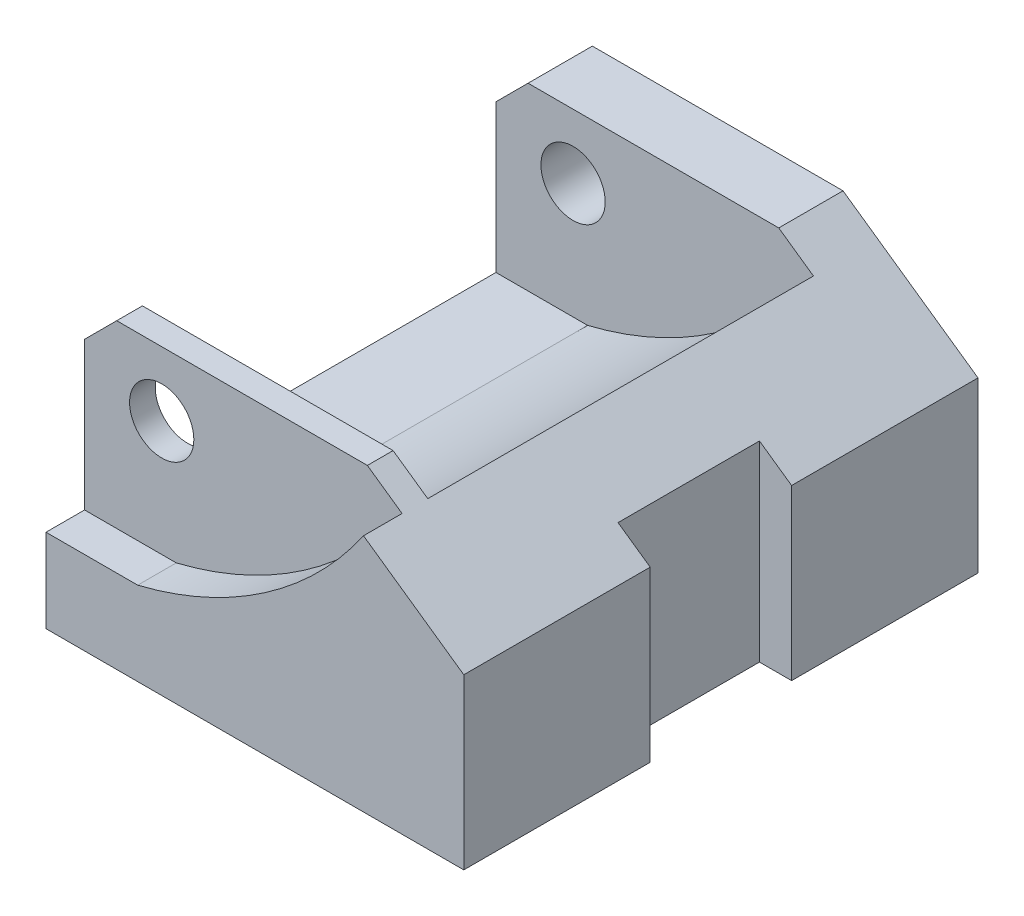
ISO-10303-21;
HEADER;
FILE_DESCRIPTION(('STEP AP214'),'2;1');
FILE_NAME('part.step','',(''),(''),'','','');
FILE_SCHEMA(('AUTOMOTIVE_DESIGN { 1 0 10303 214 1 1 1 1 }'));
ENDSEC;
DATA;
#1=APPLICATION_CONTEXT('core data for automotive mechanical design processes');
#2=APPLICATION_PROTOCOL_DEFINITION('international standard','automotive_design',2000,#1);
#3=PRODUCT_CONTEXT('',#1,'mechanical');
#4=PRODUCT('Part','Part','',(#3));
#5=PRODUCT_RELATED_PRODUCT_CATEGORY('part','',(#4));
#6=PRODUCT_DEFINITION_FORMATION('','',#4);
#7=PRODUCT_DEFINITION_CONTEXT('part definition',#1,'design');
#8=PRODUCT_DEFINITION('design','',#6,#7);
#9=PRODUCT_DEFINITION_SHAPE('','',#8);
#10=(LENGTH_UNIT() NAMED_UNIT(*) SI_UNIT(.MILLI.,.METRE.));
#11=(NAMED_UNIT(*) PLANE_ANGLE_UNIT() SI_UNIT($,.RADIAN.));
#12=(NAMED_UNIT(*) SI_UNIT($,.STERADIAN.) SOLID_ANGLE_UNIT());
#13=UNCERTAINTY_MEASURE_WITH_UNIT(LENGTH_MEASURE(1.E-05),#10,'distance_accuracy_value','');
#14=(GEOMETRIC_REPRESENTATION_CONTEXT(3) GLOBAL_UNCERTAINTY_ASSIGNED_CONTEXT((#13)) GLOBAL_UNIT_ASSIGNED_CONTEXT((#10,
#11,#12)) REPRESENTATION_CONTEXT('',''));
#15=CARTESIAN_POINT('',(0.,0.,0.));
#16=DIRECTION('',(0.,0.,1.));
#17=DIRECTION('',(1.,0.,0.));
#18=AXIS2_PLACEMENT_3D('',#15,#16,#17);
#19=CARTESIAN_POINT('',(65.,0.,40.));
#20=DIRECTION('',(-1.,0.,0.));
#21=DIRECTION('',(0.,0.,1.));
#22=AXIS2_PLACEMENT_3D('',#19,#20,#21);
#23=PLANE('',#22);
#24=DIRECTION('',(0.,-1.,0.));
#25=VECTOR('',#24,1.);
#26=CARTESIAN_POINT('',(65.,0.,11.));
#27=LINE('',#26,#25);
#28=CARTESIAN_POINT('',(65.,26.2956416975961,11.));
#29=VERTEX_POINT('',#28);
#30=CARTESIAN_POINT('',(65.,0.,11.));
#31=VERTEX_POINT('',#30);
#32=EDGE_CURVE('E176',#29,#31,#27,.T.);
#33=ORIENTED_EDGE('',*,*,#32,.F.);
#34=DIRECTION('',(0.,0.,1.));
#35=VECTOR('',#34,1.);
#36=CARTESIAN_POINT('',(65.,26.2956416975961,40.));
#37=LINE('',#36,#35);
#38=CARTESIAN_POINT('',(65.,26.2956416975961,40.));
#39=VERTEX_POINT('',#38);
#40=EDGE_CURVE('E319',#29,#39,#37,.T.);
#41=ORIENTED_EDGE('',*,*,#40,.T.);
#42=DIRECTION('',(0.,1.,0.));
#43=VECTOR('',#42,1.);
#44=CARTESIAN_POINT('',(65.,0.,40.));
#45=LINE('',#44,#43);
#46=CARTESIAN_POINT('',(65.,0.,40.));
#47=VERTEX_POINT('',#46);
#48=EDGE_CURVE('E288',#47,#39,#45,.T.);
#49=ORIENTED_EDGE('',*,*,#48,.F.);
#50=DIRECTION('',(0.,0.,-1.));
#51=VECTOR('',#50,1.);
#52=CARTESIAN_POINT('',(65.,0.,40.));
#53=LINE('',#52,#51);
#54=EDGE_CURVE('E298',#47,#31,#53,.T.);
#55=ORIENTED_EDGE('',*,*,#54,.T.);
#56=EDGE_LOOP('',(#33,#41,#49,#55));
#57=FACE_BOUND('',#56,.T.);
#58=ADVANCED_FACE('F41',(#57),#23,.F.);
#59=CARTESIAN_POINT('',(0.,41.,40.));
#60=DIRECTION('',(0.,-1.,0.));
#61=DIRECTION('',(0.,0.,-1.));
#62=AXIS2_PLACEMENT_3D('',#59,#60,#61);
#63=PLANE('',#62);
#64=DIRECTION('',(1.,0.,0.));
#65=VECTOR('',#64,1.);
#66=CARTESIAN_POINT('',(5.00000000000003,41.,-30.));
#67=LINE('',#66,#65);
#68=CARTESIAN_POINT('',(5.00000000000003,41.,-30.));
#69=VERTEX_POINT('',#68);
#70=CARTESIAN_POINT('',(43.9999999999999,41.,-30.));
#71=VERTEX_POINT('',#70);
#72=EDGE_CURVE('E218',#69,#71,#67,.T.);
#73=ORIENTED_EDGE('',*,*,#72,.T.);
#74=DIRECTION('',(0.,0.,-1.));
#75=VECTOR('',#74,1.);
#76=CARTESIAN_POINT('',(43.9999999999999,41.,40.));
#77=LINE('',#76,#75);
#78=CARTESIAN_POINT('',(43.9999999999999,41.,-40.));
#79=VERTEX_POINT('',#78);
#80=EDGE_CURVE('E315',#71,#79,#77,.T.);
#81=ORIENTED_EDGE('',*,*,#80,.T.);
#82=DIRECTION('',(-1.,0.,0.));
#83=VECTOR('',#82,1.);
#84=CARTESIAN_POINT('',(0.,41.,-40.));
#85=LINE('',#84,#83);
#86=CARTESIAN_POINT('',(5.00000000000003,41.,-40.));
#87=VERTEX_POINT('',#86);
#88=EDGE_CURVE('E283',#79,#87,#85,.T.);
#89=ORIENTED_EDGE('',*,*,#88,.T.);
#90=DIRECTION('',(0.,0.,1.));
#91=VECTOR('',#90,1.);
#92=CARTESIAN_POINT('',(5.00000000000003,41.,40.));
#93=LINE('',#92,#91);
#94=EDGE_CURVE('E307',#87,#69,#93,.T.);
#95=ORIENTED_EDGE('',*,*,#94,.T.);
#96=EDGE_LOOP('',(#73,#81,#89,#95));
#97=FACE_BOUND('',#96,.T.);
#98=ADVANCED_FACE('F357',(#97),#63,.F.);
#99=CARTESIAN_POINT('',(12.,31.,40.));
#100=DIRECTION('',(0.,0.,-1.));
#101=DIRECTION('',(-1.,0.,0.));
#102=AXIS2_PLACEMENT_3D('',#99,#100,#101);
#103=CYLINDRICAL_SURFACE('',#102,5.);
#104=CARTESIAN_POINT('',(12.,31.,-40.));
#105=DIRECTION('',(0.,0.,1.));
#106=DIRECTION('',(1.,0.,0.));
#107=AXIS2_PLACEMENT_3D('',#104,#105,#106);
#108=CIRCLE('',#107,5.);
#109=CARTESIAN_POINT('',(17.,31.,-40.));
#110=VERTEX_POINT('',#109);
#111=EDGE_CURVE('E280',#110,#110,#108,.T.);
#112=ORIENTED_EDGE('',*,*,#111,.F.);
#113=EDGE_LOOP('',(#112));
#114=FACE_BOUND('',#113,.T.);
#115=CARTESIAN_POINT('',(12.,31.,-30.));
#116=DIRECTION('',(0.,0.,1.));
#117=DIRECTION('',(1.,0.,0.));
#118=AXIS2_PLACEMENT_3D('',#115,#116,#117);
#119=CIRCLE('',#118,5.);
#120=CARTESIAN_POINT('',(17.,31.,-30.));
#121=VERTEX_POINT('',#120);
#122=EDGE_CURVE('E242',#121,#121,#119,.T.);
#123=ORIENTED_EDGE('',*,*,#122,.T.);
#124=EDGE_LOOP('',(#123));
#125=FACE_BOUND('',#124,.T.);
#126=ADVANCED_FACE('F364',(#114,#125),#103,.F.);
#127=CARTESIAN_POINT('',(0.,36.,40.));
#128=DIRECTION('',(0.707106781186546,-0.707106781186548,0.));
#129=DIRECTION('',(0.,0.,-1.));
#130=AXIS2_PLACEMENT_3D('',#127,#128,#129);
#131=PLANE('',#130);
#132=DIRECTION('',(0.,0.,-1.));
#133=VECTOR('',#132,1.);
#134=CARTESIAN_POINT('',(0.,36.,40.));
#135=LINE('',#134,#133);
#136=CARTESIAN_POINT('',(0.,36.,-30.));
#137=VERTEX_POINT('',#136);
#138=CARTESIAN_POINT('',(0.,36.,-40.));
#139=VERTEX_POINT('',#138);
#140=EDGE_CURVE('E301',#137,#139,#135,.T.);
#141=ORIENTED_EDGE('',*,*,#140,.F.);
#142=DIRECTION('',(0.707106781186548,0.707106781186546,0.));
#143=VECTOR('',#142,1.);
#144=CARTESIAN_POINT('',(0.,36.,-30.));
#145=LINE('',#144,#143);
#146=EDGE_CURVE('E219',#137,#69,#145,.T.);
#147=ORIENTED_EDGE('',*,*,#146,.T.);
#148=ORIENTED_EDGE('',*,*,#94,.F.);
#149=DIRECTION('',(-0.707106781186549,-0.707106781186547,0.));
#150=VECTOR('',#149,1.);
#151=CARTESIAN_POINT('',(-18.,18.,-40.));
#152=LINE('',#151,#150);
#153=EDGE_CURVE('E304',#139,#87,#152,.F.);
#154=ORIENTED_EDGE('',*,*,#153,.F.);
#155=EDGE_LOOP('',(#141,#147,#148,#154));
#156=FACE_BOUND('',#155,.T.);
#157=ADVANCED_FACE('F365',(#156),#131,.F.);
#158=CARTESIAN_POINT('',(0.,0.,40.));
#159=DIRECTION('',(1.,0.,0.));
#160=DIRECTION('',(0.,0.,-1.));
#161=AXIS2_PLACEMENT_3D('',#158,#159,#160);
#162=PLANE('',#161);
#163=DIRECTION('',(0.,1.,0.));
#164=VECTOR('',#163,1.);
#165=CARTESIAN_POINT('',(0.,13.,-30.));
#166=LINE('',#165,#164);
#167=CARTESIAN_POINT('',(0.,13.,-30.));
#168=VERTEX_POINT('',#167);
#169=EDGE_CURVE('E214',#168,#137,#166,.T.);
#170=ORIENTED_EDGE('',*,*,#169,.T.);
#171=ORIENTED_EDGE('',*,*,#140,.T.);
#172=DIRECTION('',(0.,-1.,0.));
#173=VECTOR('',#172,1.);
#174=CARTESIAN_POINT('',(0.,0.,-40.));
#175=LINE('',#174,#173);
#176=CARTESIAN_POINT('',(0.,0.,-40.));
#177=VERTEX_POINT('',#176);
#178=EDGE_CURVE('E278',#139,#177,#175,.T.);
#179=ORIENTED_EDGE('',*,*,#178,.T.);
#180=DIRECTION('',(0.,0.,-1.));
#181=VECTOR('',#180,1.);
#182=CARTESIAN_POINT('',(0.,0.,40.));
#183=LINE('',#182,#181);
#184=CARTESIAN_POINT('',(0.,0.,40.));
#185=VERTEX_POINT('',#184);
#186=EDGE_CURVE('E296',#185,#177,#183,.T.);
#187=ORIENTED_EDGE('',*,*,#186,.F.);
#188=DIRECTION('',(0.,-1.,0.));
#189=VECTOR('',#188,1.);
#190=CARTESIAN_POINT('',(0.,0.,40.));
#191=LINE('',#190,#189);
#192=CARTESIAN_POINT('',(0.,13.,40.));
#193=VERTEX_POINT('',#192);
#194=EDGE_CURVE('E284',#193,#185,#191,.T.);
#195=ORIENTED_EDGE('',*,*,#194,.F.);
#196=DIRECTION('',(0.,0.,1.));
#197=VECTOR('',#196,1.);
#198=CARTESIAN_POINT('',(0.,13.,34.));
#199=LINE('',#198,#197);
#200=CARTESIAN_POINT('',(0.,13.,34.));
#201=VERTEX_POINT('',#200);
#202=EDGE_CURVE('E263',#201,#193,#199,.T.);
#203=ORIENTED_EDGE('',*,*,#202,.F.);
#204=DIRECTION('',(0.,-1.,0.));
#205=VECTOR('',#204,1.);
#206=CARTESIAN_POINT('',(0.,13.,34.));
#207=LINE('',#206,#205);
#208=CARTESIAN_POINT('',(0.,36.,34.));
#209=VERTEX_POINT('',#208);
#210=EDGE_CURVE('E247',#209,#201,#207,.T.);
#211=ORIENTED_EDGE('',*,*,#210,.F.);
#212=CARTESIAN_POINT('',(0.,36.,30.));
#213=VERTEX_POINT('',#212);
#214=EDGE_CURVE('E305',#209,#213,#135,.T.);
#215=ORIENTED_EDGE('',*,*,#214,.T.);
#216=DIRECTION('',(0.,1.,0.));
#217=VECTOR('',#216,1.);
#218=CARTESIAN_POINT('',(0.,13.,30.));
#219=LINE('',#218,#217);
#220=CARTESIAN_POINT('',(0.,13.,30.));
#221=VERTEX_POINT('',#220);
#222=EDGE_CURVE('E229',#221,#213,#219,.T.);
#223=ORIENTED_EDGE('',*,*,#222,.F.);
#224=DIRECTION('',(0.,0.,1.));
#225=VECTOR('',#224,1.);
#226=CARTESIAN_POINT('',(0.,13.,-30.));
#227=LINE('',#226,#225);
#228=EDGE_CURVE('E224',#168,#221,#227,.T.);
#229=ORIENTED_EDGE('',*,*,#228,.F.);
#230=EDGE_LOOP('',(#170,#171,#179,#187,#195,#203,#211,#215,#223,#229));
#231=FACE_BOUND('',#230,.T.);
#232=ADVANCED_FACE('F341',(#231),#162,.F.);
#233=CARTESIAN_POINT('',(43.9999999999999,41.,40.));
#234=DIRECTION('',(-0.573576436351044,-0.819152044288993,0.));
#235=DIRECTION('',(0.,0.,-1.));
#236=AXIS2_PLACEMENT_3D('',#233,#234,#235);
#237=PLANE('',#236);
#238=DIRECTION('',(0.819152044288993,-0.573576436351044,0.));
#239=VECTOR('',#238,1.);
#240=CARTESIAN_POINT('',(43.9999999999999,41.,-11.));
#241=LINE('',#240,#239);
#242=CARTESIAN_POINT('',(65.,26.2956416975961,-11.));
#243=VERTEX_POINT('',#242);
#244=CARTESIAN_POINT('',(60.,29.7966793886446,-11.));
#245=VERTEX_POINT('',#244);
#246=EDGE_CURVE('E196',#243,#245,#241,.F.);
#247=ORIENTED_EDGE('',*,*,#246,.F.);
#248=CARTESIAN_POINT('',(65.,26.2956416975961,-40.));
#249=VERTEX_POINT('',#248);
#250=EDGE_CURVE('E316',#249,#243,#37,.T.);
#251=ORIENTED_EDGE('',*,*,#250,.F.);
#252=DIRECTION('',(-0.819152044288993,0.573576436351044,0.));
#253=VECTOR('',#252,1.);
#254=CARTESIAN_POINT('',(33.7392555729462,48.1846505954662,-40.));
#255=LINE('',#254,#253);
#256=EDGE_CURVE('E317',#79,#249,#255,.F.);
#257=ORIENTED_EDGE('',*,*,#256,.F.);
#258=ORIENTED_EDGE('',*,*,#80,.F.);
#259=DIRECTION('',(0.819152044288991,-0.573576436351047,0.));
#260=VECTOR('',#259,1.);
#261=CARTESIAN_POINT('',(43.9999999999999,41.,-30.));
#262=LINE('',#261,#260);
#263=CARTESIAN_POINT('',(49.3966026023433,37.2212581771169,-30.));
#264=VERTEX_POINT('',#263);
#265=EDGE_CURVE('E205',#71,#264,#262,.T.);
#266=ORIENTED_EDGE('',*,*,#265,.T.);
#267=DIRECTION('',(0.,0.,1.));
#268=VECTOR('',#267,1.);
#269=CARTESIAN_POINT('',(49.3966026023433,37.2212581771169,-30.));
#270=LINE('',#269,#268);
#271=CARTESIAN_POINT('',(49.3966026023433,37.2212581771169,30.));
#272=VERTEX_POINT('',#271);
#273=EDGE_CURVE('E238',#264,#272,#270,.T.);
#274=ORIENTED_EDGE('',*,*,#273,.T.);
#275=DIRECTION('',(0.819152044288991,-0.573576436351047,0.));
#276=VECTOR('',#275,1.);
#277=CARTESIAN_POINT('',(43.9999999999999,41.,30.));
#278=LINE('',#277,#276);
#279=CARTESIAN_POINT('',(43.9999999999999,41.,30.));
#280=VERTEX_POINT('',#279);
#281=EDGE_CURVE('E202',#280,#272,#278,.T.);
#282=ORIENTED_EDGE('',*,*,#281,.F.);
#283=CARTESIAN_POINT('',(43.9999999999999,41.,34.));
#284=VERTEX_POINT('',#283);
#285=EDGE_CURVE('E312',#284,#280,#77,.T.);
#286=ORIENTED_EDGE('',*,*,#285,.F.);
#287=DIRECTION('',(-0.819152044288993,0.573576436351044,0.));
#288=VECTOR('',#287,1.);
#289=CARTESIAN_POINT('',(43.9999999999999,41.,34.));
#290=LINE('',#289,#288);
#291=CARTESIAN_POINT('',(49.3966026023433,37.221258177117,34.));
#292=VERTEX_POINT('',#291);
#293=EDGE_CURVE('E260',#292,#284,#290,.T.);
#294=ORIENTED_EDGE('',*,*,#293,.F.);
#295=DIRECTION('',(0.,0.,1.));
#296=VECTOR('',#295,1.);
#297=CARTESIAN_POINT('',(49.3966026023433,37.221258177117,34.));
#298=LINE('',#297,#296);
#299=CARTESIAN_POINT('',(49.3966026023433,37.221258177117,40.));
#300=VERTEX_POINT('',#299);
#301=EDGE_CURVE('E267',#292,#300,#298,.T.);
#302=ORIENTED_EDGE('',*,*,#301,.T.);
#303=DIRECTION('',(0.819152044288993,-0.573576436351044,0.));
#304=VECTOR('',#303,1.);
#305=CARTESIAN_POINT('',(43.9999999999999,41.,40.));
#306=LINE('',#305,#304);
#307=EDGE_CURVE('E325',#39,#300,#306,.F.);
#308=ORIENTED_EDGE('',*,*,#307,.F.);
#309=ORIENTED_EDGE('',*,*,#40,.F.);
#310=DIRECTION('',(0.819152044288993,-0.573576436351044,0.));
#311=VECTOR('',#310,1.);
#312=CARTESIAN_POINT('',(43.9999999999999,41.,11.));
#313=LINE('',#312,#311);
#314=CARTESIAN_POINT('',(60.,29.7966793886446,11.));
#315=VERTEX_POINT('',#314);
#316=EDGE_CURVE('E60',#29,#315,#313,.F.);
#317=ORIENTED_EDGE('',*,*,#316,.T.);
#318=DIRECTION('',(0.,0.,-1.));
#319=VECTOR('',#318,1.);
#320=CARTESIAN_POINT('',(60.,29.7966793886446,40.));
#321=LINE('',#320,#319);
#322=EDGE_CURVE('E187',#245,#315,#321,.F.);
#323=ORIENTED_EDGE('',*,*,#322,.F.);
#324=EDGE_LOOP('',(#247,#251,#257,#258,#266,#274,#282,#286,#294,#302,#308,#309,#317,#323));
#325=FACE_BOUND('',#324,.T.);
#326=ADVANCED_FACE('F42',(#325),#237,.F.);
#327=ORIENTED_EDGE('',*,*,#285,.T.);
#328=DIRECTION('',(1.,0.,0.));
#329=VECTOR('',#328,1.);
#330=CARTESIAN_POINT('',(5.00000000000003,41.,30.));
#331=LINE('',#330,#329);
#332=CARTESIAN_POINT('',(5.00000000000003,41.,30.));
#333=VERTEX_POINT('',#332);
#334=EDGE_CURVE('E63',#333,#280,#331,.T.);
#335=ORIENTED_EDGE('',*,*,#334,.F.);
#336=CARTESIAN_POINT('',(5.00000000000003,41.,34.));
#337=VERTEX_POINT('',#336);
#338=EDGE_CURVE('E308',#333,#337,#93,.T.);
#339=ORIENTED_EDGE('',*,*,#338,.T.);
#340=DIRECTION('',(-1.,0.,0.));
#341=VECTOR('',#340,1.);
#342=CARTESIAN_POINT('',(5.00000000000003,41.,34.));
#343=LINE('',#342,#341);
#344=EDGE_CURVE('E256',#284,#337,#343,.T.);
#345=ORIENTED_EDGE('',*,*,#344,.F.);
#346=EDGE_LOOP('',(#327,#335,#339,#345));
#347=FACE_BOUND('',#346,.T.);
#348=ADVANCED_FACE('F383',(#347),#63,.F.);
#349=CARTESIAN_POINT('',(12.,31.,30.));
#350=DIRECTION('',(0.,0.,1.));
#351=DIRECTION('',(1.,0.,0.));
#352=AXIS2_PLACEMENT_3D('',#349,#350,#351);
#353=CIRCLE('',#352,5.);
#354=CARTESIAN_POINT('',(17.,31.,30.));
#355=VERTEX_POINT('',#354);
#356=EDGE_CURVE('E241',#355,#355,#353,.T.);
#357=ORIENTED_EDGE('',*,*,#356,.F.);
#358=EDGE_LOOP('',(#357));
#359=FACE_BOUND('',#358,.T.);
#360=CARTESIAN_POINT('',(12.,31.,34.));
#361=DIRECTION('',(0.,0.,1.));
#362=DIRECTION('',(1.,0.,0.));
#363=AXIS2_PLACEMENT_3D('',#360,#361,#362);
#364=CIRCLE('',#363,5.);
#365=CARTESIAN_POINT('',(17.,31.,34.));
#366=VERTEX_POINT('',#365);
#367=EDGE_CURVE('E272',#366,#366,#364,.T.);
#368=ORIENTED_EDGE('',*,*,#367,.T.);
#369=EDGE_LOOP('',(#368));
#370=FACE_BOUND('',#369,.T.);
#371=ADVANCED_FACE('F373',(#359,#370),#103,.F.);
#372=DIRECTION('',(0.707106781186548,0.707106781186546,0.));
#373=VECTOR('',#372,1.);
#374=CARTESIAN_POINT('',(0.,36.,30.));
#375=LINE('',#374,#373);
#376=EDGE_CURVE('E235',#213,#333,#375,.T.);
#377=ORIENTED_EDGE('',*,*,#376,.F.);
#378=ORIENTED_EDGE('',*,*,#214,.F.);
#379=DIRECTION('',(-0.707106781186548,-0.707106781186546,0.));
#380=VECTOR('',#379,1.);
#381=CARTESIAN_POINT('',(0.,36.,34.));
#382=LINE('',#381,#380);
#383=EDGE_CURVE('E261',#337,#209,#382,.T.);
#384=ORIENTED_EDGE('',*,*,#383,.F.);
#385=ORIENTED_EDGE('',*,*,#338,.F.);
#386=EDGE_LOOP('',(#377,#378,#384,#385));
#387=FACE_BOUND('',#386,.T.);
#388=ADVANCED_FACE('F362',(#387),#131,.F.);
#389=CARTESIAN_POINT('',(0.,0.,40.));
#390=DIRECTION('',(0.,0.,-1.));
#391=DIRECTION('',(-1.,0.,0.));
#392=AXIS2_PLACEMENT_3D('',#389,#390,#391);
#393=PLANE('',#392);
#394=ORIENTED_EDGE('',*,*,#307,.T.);
#395=CARTESIAN_POINT('',(0.,71.2796734565478,40.));
#396=DIRECTION('',(0.,0.,1.));
#397=DIRECTION('',(1.,0.,0.));
#398=AXIS2_PLACEMENT_3D('',#395,#396,#397);
#399=CIRCLE('',#398,60.);
#400=CARTESIAN_POINT('',(14.2646297462696,13.,40.));
#401=VERTEX_POINT('',#400);
#402=EDGE_CURVE('E255',#401,#300,#399,.T.);
#403=ORIENTED_EDGE('',*,*,#402,.F.);
#404=DIRECTION('',(1.,0.,0.));
#405=VECTOR('',#404,1.);
#406=CARTESIAN_POINT('',(0.,13.,40.));
#407=LINE('',#406,#405);
#408=EDGE_CURVE('E250',#193,#401,#407,.T.);
#409=ORIENTED_EDGE('',*,*,#408,.F.);
#410=ORIENTED_EDGE('',*,*,#194,.T.);
#411=DIRECTION('',(1.,0.,0.));
#412=VECTOR('',#411,1.);
#413=CARTESIAN_POINT('',(0.,0.,40.));
#414=LINE('',#413,#412);
#415=EDGE_CURVE('E285',#185,#47,#414,.T.);
#416=ORIENTED_EDGE('',*,*,#415,.T.);
#417=ORIENTED_EDGE('',*,*,#48,.T.);
#418=EDGE_LOOP('',(#394,#403,#409,#410,#416,#417));
#419=FACE_BOUND('',#418,.T.);
#420=ADVANCED_FACE('F340',(#419),#393,.F.);
#421=CARTESIAN_POINT('',(0.,0.,-40.));
#422=DIRECTION('',(0.,0.,-1.));
#423=DIRECTION('',(-1.,0.,0.));
#424=AXIS2_PLACEMENT_3D('',#421,#422,#423);
#425=PLANE('',#424);
#426=ORIENTED_EDGE('',*,*,#88,.F.);
#427=ORIENTED_EDGE('',*,*,#256,.T.);
#428=DIRECTION('',(0.,1.,0.));
#429=VECTOR('',#428,1.);
#430=CARTESIAN_POINT('',(65.,0.,-40.));
#431=LINE('',#430,#429);
#432=CARTESIAN_POINT('',(65.,0.,-40.));
#433=VERTEX_POINT('',#432);
#434=EDGE_CURVE('E292',#433,#249,#431,.T.);
#435=ORIENTED_EDGE('',*,*,#434,.F.);
#436=DIRECTION('',(1.,0.,0.));
#437=VECTOR('',#436,1.);
#438=CARTESIAN_POINT('',(0.,0.,-40.));
#439=LINE('',#438,#437);
#440=EDGE_CURVE('E286',#177,#433,#439,.T.);
#441=ORIENTED_EDGE('',*,*,#440,.F.);
#442=ORIENTED_EDGE('',*,*,#178,.F.);
#443=ORIENTED_EDGE('',*,*,#153,.T.);
#444=EDGE_LOOP('',(#426,#427,#435,#441,#442,#443));
#445=FACE_BOUND('',#444,.T.);
#446=ORIENTED_EDGE('',*,*,#111,.T.);
#447=EDGE_LOOP('',(#446));
#448=FACE_BOUND('',#447,.T.);
#449=ADVANCED_FACE('F352',(#445,#448),#425,.T.);
#450=CARTESIAN_POINT('',(0.,0.,40.));
#451=DIRECTION('',(0.,1.,0.));
#452=DIRECTION('',(0.,0.,1.));
#453=AXIS2_PLACEMENT_3D('',#450,#451,#452);
#454=PLANE('',#453);
#455=CARTESIAN_POINT('',(65.,0.,-11.));
#456=VERTEX_POINT('',#455);
#457=EDGE_CURVE('E191',#456,#433,#53,.T.);
#458=ORIENTED_EDGE('',*,*,#457,.F.);
#459=DIRECTION('',(-1.,0.,0.));
#460=VECTOR('',#459,1.);
#461=CARTESIAN_POINT('',(0.,0.,-11.));
#462=LINE('',#461,#460);
#463=CARTESIAN_POINT('',(60.,0.,-11.));
#464=VERTEX_POINT('',#463);
#465=EDGE_CURVE('E195',#456,#464,#462,.T.);
#466=ORIENTED_EDGE('',*,*,#465,.T.);
#467=DIRECTION('',(0.,0.,1.));
#468=VECTOR('',#467,1.);
#469=CARTESIAN_POINT('',(60.,0.,40.));
#470=LINE('',#469,#468);
#471=CARTESIAN_POINT('',(60.,0.,11.));
#472=VERTEX_POINT('',#471);
#473=EDGE_CURVE('E11',#464,#472,#470,.T.);
#474=ORIENTED_EDGE('',*,*,#473,.T.);
#475=DIRECTION('',(-1.,0.,0.));
#476=VECTOR('',#475,1.);
#477=CARTESIAN_POINT('',(0.,0.,11.));
#478=LINE('',#477,#476);
#479=EDGE_CURVE('E175',#31,#472,#478,.T.);
#480=ORIENTED_EDGE('',*,*,#479,.F.);
#481=ORIENTED_EDGE('',*,*,#54,.F.);
#482=ORIENTED_EDGE('',*,*,#415,.F.);
#483=ORIENTED_EDGE('',*,*,#186,.T.);
#484=ORIENTED_EDGE('',*,*,#440,.T.);
#485=EDGE_LOOP('',(#458,#466,#474,#480,#481,#482,#483,#484));
#486=FACE_BOUND('',#485,.T.);
#487=ADVANCED_FACE('F192',(#486),#454,.F.);
#488=ORIENTED_EDGE('',*,*,#250,.T.);
#489=DIRECTION('',(0.,-1.,0.));
#490=VECTOR('',#489,1.);
#491=CARTESIAN_POINT('',(65.,0.,-11.));
#492=LINE('',#491,#490);
#493=EDGE_CURVE('E49',#243,#456,#492,.T.);
#494=ORIENTED_EDGE('',*,*,#493,.T.);
#495=ORIENTED_EDGE('',*,*,#457,.T.);
#496=ORIENTED_EDGE('',*,*,#434,.T.);
#497=EDGE_LOOP('',(#488,#494,#495,#496));
#498=FACE_BOUND('',#497,.T.);
#499=ADVANCED_FACE('F329',(#498),#23,.F.);
#500=CARTESIAN_POINT('',(0.,71.2796734565478,34.));
#501=DIRECTION('',(0.,0.,1.));
#502=DIRECTION('',(1.,0.,0.));
#503=AXIS2_PLACEMENT_3D('',#500,#501,#502);
#504=CYLINDRICAL_SURFACE('',#503,60.);
#505=ORIENTED_EDGE('',*,*,#402,.T.);
#506=ORIENTED_EDGE('',*,*,#301,.F.);
#507=CARTESIAN_POINT('',(0.,71.2796734565478,34.));
#508=DIRECTION('',(0.,0.,1.));
#509=DIRECTION('',(1.,0.,0.));
#510=AXIS2_PLACEMENT_3D('',#507,#508,#509);
#511=CIRCLE('',#510,60.);
#512=CARTESIAN_POINT('',(14.2646297462696,13.,34.));
#513=VERTEX_POINT('',#512);
#514=EDGE_CURVE('E253',#513,#292,#511,.T.);
#515=ORIENTED_EDGE('',*,*,#514,.F.);
#516=DIRECTION('',(0.,0.,1.));
#517=VECTOR('',#516,1.);
#518=CARTESIAN_POINT('',(14.2646297462696,13.,34.));
#519=LINE('',#518,#517);
#520=EDGE_CURVE('E275',#513,#401,#519,.T.);
#521=ORIENTED_EDGE('',*,*,#520,.T.);
#522=EDGE_LOOP('',(#505,#506,#515,#521));
#523=FACE_BOUND('',#522,.T.);
#524=ADVANCED_FACE('F389',(#523),#504,.F.);
#525=CARTESIAN_POINT('',(0.,13.,34.));
#526=DIRECTION('',(0.,-1.,0.));
#527=DIRECTION('',(1.,0.,0.));
#528=AXIS2_PLACEMENT_3D('',#525,#526,#527);
#529=PLANE('',#528);
#530=ORIENTED_EDGE('',*,*,#408,.T.);
#531=ORIENTED_EDGE('',*,*,#520,.F.);
#532=DIRECTION('',(1.,0.,0.));
#533=VECTOR('',#532,1.);
#534=CARTESIAN_POINT('',(0.,13.,34.));
#535=LINE('',#534,#533);
#536=EDGE_CURVE('E252',#201,#513,#535,.T.);
#537=ORIENTED_EDGE('',*,*,#536,.F.);
#538=ORIENTED_EDGE('',*,*,#202,.T.);
#539=EDGE_LOOP('',(#530,#531,#537,#538));
#540=FACE_BOUND('',#539,.T.);
#541=ADVANCED_FACE('F393',(#540),#529,.F.);
#542=CARTESIAN_POINT('',(0.,71.2796734565478,34.));
#543=DIRECTION('',(0.,0.,1.));
#544=DIRECTION('',(1.,0.,0.));
#545=AXIS2_PLACEMENT_3D('',#542,#543,#544);
#546=PLANE('',#545);
#547=ORIENTED_EDGE('',*,*,#367,.F.);
#548=EDGE_LOOP('',(#547));
#549=FACE_BOUND('',#548,.T.);
#550=ORIENTED_EDGE('',*,*,#210,.T.);
#551=ORIENTED_EDGE('',*,*,#536,.T.);
#552=ORIENTED_EDGE('',*,*,#514,.T.);
#553=ORIENTED_EDGE('',*,*,#293,.T.);
#554=ORIENTED_EDGE('',*,*,#344,.T.);
#555=ORIENTED_EDGE('',*,*,#383,.T.);
#556=EDGE_LOOP('',(#550,#551,#552,#553,#554,#555));
#557=FACE_BOUND('',#556,.T.);
#558=ADVANCED_FACE('F431',(#549,#557),#546,.T.);
#559=CARTESIAN_POINT('',(0.,71.2796734565478,-30.));
#560=DIRECTION('',(0.,0.,1.));
#561=DIRECTION('',(1.,0.,0.));
#562=AXIS2_PLACEMENT_3D('',#559,#560,#561);
#563=CYLINDRICAL_SURFACE('',#562,60.);
#564=CARTESIAN_POINT('',(0.,71.2796734565478,30.));
#565=DIRECTION('',(0.,0.,1.));
#566=DIRECTION('',(1.,0.,0.));
#567=AXIS2_PLACEMENT_3D('',#564,#565,#566);
#568=CIRCLE('',#567,60.);
#569=CARTESIAN_POINT('',(14.2646297462697,13.,30.));
#570=VERTEX_POINT('',#569);
#571=EDGE_CURVE('E225',#570,#272,#568,.T.);
#572=ORIENTED_EDGE('',*,*,#571,.T.);
#573=ORIENTED_EDGE('',*,*,#273,.F.);
#574=CARTESIAN_POINT('',(0.,71.2796734565478,-30.));
#575=DIRECTION('',(0.,0.,1.));
#576=DIRECTION('',(1.,0.,0.));
#577=AXIS2_PLACEMENT_3D('',#574,#575,#576);
#578=CIRCLE('',#577,60.);
#579=CARTESIAN_POINT('',(14.2646297462697,13.,-30.));
#580=VERTEX_POINT('',#579);
#581=EDGE_CURVE('E210',#580,#264,#578,.T.);
#582=ORIENTED_EDGE('',*,*,#581,.F.);
#583=DIRECTION('',(0.,0.,1.));
#584=VECTOR('',#583,1.);
#585=CARTESIAN_POINT('',(14.2646297462697,13.,-30.));
#586=LINE('',#585,#584);
#587=EDGE_CURVE('E236',#580,#570,#586,.T.);
#588=ORIENTED_EDGE('',*,*,#587,.T.);
#589=EDGE_LOOP('',(#572,#573,#582,#588));
#590=FACE_BOUND('',#589,.T.);
#591=ADVANCED_FACE('F420',(#590),#563,.F.);
#592=CARTESIAN_POINT('',(0.,13.,-30.));
#593=DIRECTION('',(0.,-1.,0.));
#594=DIRECTION('',(1.,0.,0.));
#595=AXIS2_PLACEMENT_3D('',#592,#593,#594);
#596=PLANE('',#595);
#597=DIRECTION('',(1.,0.,0.));
#598=VECTOR('',#597,1.);
#599=CARTESIAN_POINT('',(0.,13.,30.));
#600=LINE('',#599,#598);
#601=EDGE_CURVE('E227',#221,#570,#600,.T.);
#602=ORIENTED_EDGE('',*,*,#601,.T.);
#603=ORIENTED_EDGE('',*,*,#587,.F.);
#604=DIRECTION('',(1.,0.,0.));
#605=VECTOR('',#604,1.);
#606=CARTESIAN_POINT('',(0.,13.,-30.));
#607=LINE('',#606,#605);
#608=EDGE_CURVE('E208',#168,#580,#607,.T.);
#609=ORIENTED_EDGE('',*,*,#608,.F.);
#610=ORIENTED_EDGE('',*,*,#228,.T.);
#611=EDGE_LOOP('',(#602,#603,#609,#610));
#612=FACE_BOUND('',#611,.T.);
#613=ADVANCED_FACE('F421',(#612),#596,.F.);
#614=CARTESIAN_POINT('',(0.,71.2796734565478,-30.));
#615=DIRECTION('',(0.,0.,1.));
#616=DIRECTION('',(1.,0.,0.));
#617=AXIS2_PLACEMENT_3D('',#614,#615,#616);
#618=PLANE('',#617);
#619=ORIENTED_EDGE('',*,*,#122,.F.);
#620=EDGE_LOOP('',(#619));
#621=FACE_BOUND('',#620,.T.);
#622=ORIENTED_EDGE('',*,*,#265,.F.);
#623=ORIENTED_EDGE('',*,*,#72,.F.);
#624=ORIENTED_EDGE('',*,*,#146,.F.);
#625=ORIENTED_EDGE('',*,*,#169,.F.);
#626=ORIENTED_EDGE('',*,*,#608,.T.);
#627=ORIENTED_EDGE('',*,*,#581,.T.);
#628=EDGE_LOOP('',(#622,#623,#624,#625,#626,#627));
#629=FACE_BOUND('',#628,.T.);
#630=ADVANCED_FACE('F359',(#621,#629),#618,.T.);
#631=CARTESIAN_POINT('',(0.,71.2796734565478,30.));
#632=DIRECTION('',(0.,0.,1.));
#633=DIRECTION('',(1.,0.,0.));
#634=AXIS2_PLACEMENT_3D('',#631,#632,#633);
#635=PLANE('',#634);
#636=ORIENTED_EDGE('',*,*,#356,.T.);
#637=EDGE_LOOP('',(#636));
#638=FACE_BOUND('',#637,.T.);
#639=ORIENTED_EDGE('',*,*,#281,.T.);
#640=ORIENTED_EDGE('',*,*,#571,.F.);
#641=ORIENTED_EDGE('',*,*,#601,.F.);
#642=ORIENTED_EDGE('',*,*,#222,.T.);
#643=ORIENTED_EDGE('',*,*,#376,.T.);
#644=ORIENTED_EDGE('',*,*,#334,.T.);
#645=EDGE_LOOP('',(#639,#640,#641,#642,#643,#644));
#646=FACE_BOUND('',#645,.T.);
#647=ADVANCED_FACE('F418',(#638,#646),#635,.F.);
#648=CARTESIAN_POINT('',(60.,-169.,-11.));
#649=DIRECTION('',(-1.,0.,0.));
#650=DIRECTION('',(0.,0.,1.));
#651=AXIS2_PLACEMENT_3D('',#648,#649,#650);
#652=PLANE('',#651);
#653=ORIENTED_EDGE('',*,*,#322,.T.);
#654=DIRECTION('',(0.,1.,0.));
#655=VECTOR('',#654,1.);
#656=CARTESIAN_POINT('',(60.,-169.,11.));
#657=LINE('',#656,#655);
#658=EDGE_CURVE('E174',#472,#315,#657,.T.);
#659=ORIENTED_EDGE('',*,*,#658,.F.);
#660=ORIENTED_EDGE('',*,*,#473,.F.);
#661=DIRECTION('',(0.,1.,0.));
#662=VECTOR('',#661,1.);
#663=CARTESIAN_POINT('',(60.,-169.,-11.));
#664=LINE('',#663,#662);
#665=EDGE_CURVE('E190',#464,#245,#664,.T.);
#666=ORIENTED_EDGE('',*,*,#665,.T.);
#667=EDGE_LOOP('',(#653,#659,#660,#666));
#668=FACE_BOUND('',#667,.T.);
#669=ADVANCED_FACE('F185',(#668),#652,.F.);
#670=CARTESIAN_POINT('',(65.,-169.,-11.));
#671=DIRECTION('',(0.,0.,-1.));
#672=DIRECTION('',(-1.,0.,0.));
#673=AXIS2_PLACEMENT_3D('',#670,#671,#672);
#674=PLANE('',#673);
#675=ORIENTED_EDGE('',*,*,#246,.T.);
#676=ORIENTED_EDGE('',*,*,#665,.F.);
#677=ORIENTED_EDGE('',*,*,#465,.F.);
#678=ORIENTED_EDGE('',*,*,#493,.F.);
#679=EDGE_LOOP('',(#675,#676,#677,#678));
#680=FACE_BOUND('',#679,.T.);
#681=ADVANCED_FACE('F328',(#680),#674,.F.);
#682=CARTESIAN_POINT('',(65.,-169.,11.));
#683=DIRECTION('',(0.,0.,-1.));
#684=DIRECTION('',(-1.,0.,0.));
#685=AXIS2_PLACEMENT_3D('',#682,#683,#684);
#686=PLANE('',#685);
#687=ORIENTED_EDGE('',*,*,#32,.T.);
#688=ORIENTED_EDGE('',*,*,#479,.T.);
#689=ORIENTED_EDGE('',*,*,#658,.T.);
#690=ORIENTED_EDGE('',*,*,#316,.F.);
#691=EDGE_LOOP('',(#687,#688,#689,#690));
#692=FACE_BOUND('',#691,.T.);
#693=ADVANCED_FACE('F172',(#692),#686,.T.);
#694=CLOSED_SHELL('',(#58,#98,#126,#157,#232,#326,#348,#371,#388,#420,#449,#487,#499,#524,#541,
#558,#591,#613,#630,#647,#669,#681,#693));
#695=MANIFOLD_SOLID_BREP('B2',#694);
#696=ADVANCED_BREP_SHAPE_REPRESENTATION('',(#18,#695),#14);
#697=SHAPE_DEFINITION_REPRESENTATION(#9,#696);
ENDSEC;
END-ISO-10303-21;
